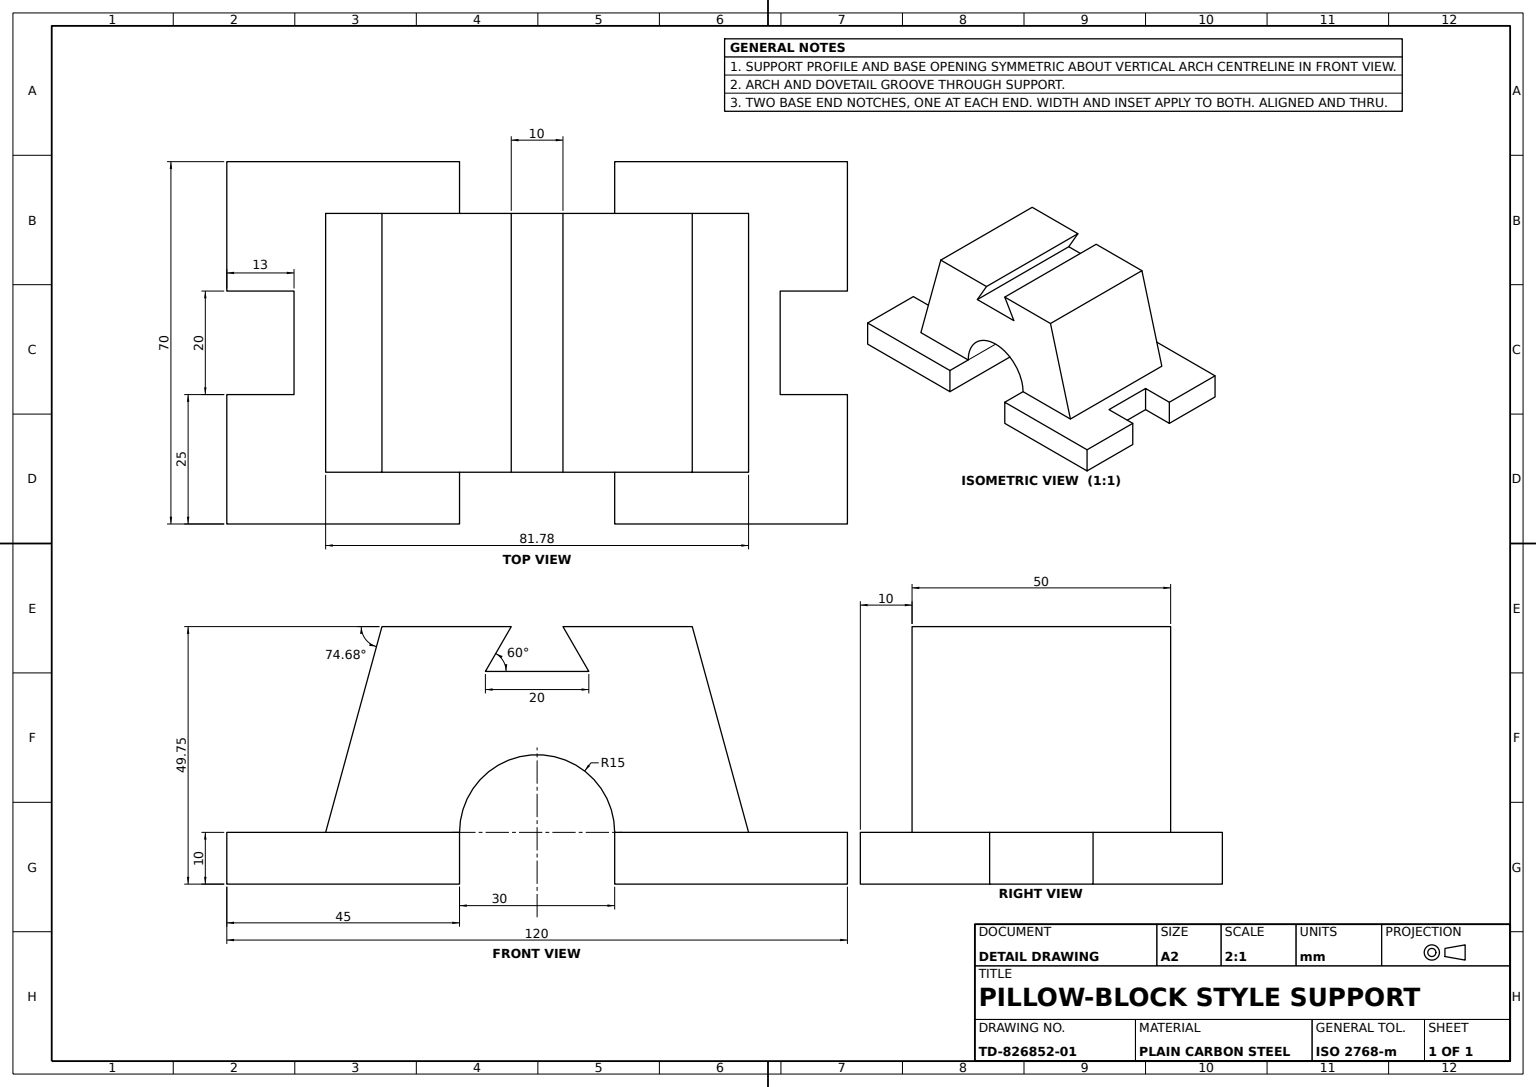
from build123d import *

# Parameters (mm, degrees)
BASE_PLATE_10MM_DEPTH         = 10
SUPPORT_BLOCK_50MM_DEPTH      = 25
SUPPORT_BLOCK_50MM_DEPTH_BACK = 25
ARCH_THROUGH_CUT_DEPTH        = 35
ARCH_THROUGH_CUT_DEPTH_BACK   = 35
UPPER_BOSS_SKETCH_W           = 20
UPPER_BOSS_SKETCH_H           = 10
UPPER_BOSS_3MM_DEPTH          = 3
BASE_PAD_SKETCH_W             = 20
BASE_PAD_SKETCH_H             = 10
BASE_PAD_4_19MM_DEPTH         = 4.19


with BuildPart() as part:
    # Base Plate Sketch → Base Plate 10mm (new body)
    with BuildSketch(Plane(origin=(0, 0, 0), x_dir=(1, 0, 0), z_dir=(0, 1, 0))):
        Polygon((60, 10), (42.8083356, 10), (42.8083356, -10), (60, -10), (60, -35), (-60, -35), (-60, -10), (-44.9850804, -10), (-44.9850804, 10), (-60, 10), (-60, 35), (60, 35), align=None)
    extrude(amount=BASE_PLATE_10MM_DEPTH)

    # Support Block Profile → Support Block 50mm (add, two sides: drawn at the far end of the back side and taken through both)
    with BuildSketch(Plane.XY.offset(-SUPPORT_BLOCK_50MM_DEPTH_BACK)):
        with BuildLine():
            Line((-40.889682702, 10), (-15, 10))
            ThreePointArc((-15, 10), (0, 25), (15, 10))
            Line((15, 10), (40.889682702, 10))
            Line((40.889682702, 10), (30, 49.749371855))
            Line((30, 49.749371855), (5, 49.749371855))
            Line((5, 49.749371855), (10, 41.089117817))
            Line((10, 41.089117817), (-10, 41.089117817))
            Line((-10, 41.089117817), (-5, 49.749371855))
            Line((-5, 49.749371855), (-30, 49.749371855))
            Line((-30, 49.749371855), (-40.889682702, 10))
        make_face()
        with BuildLine():
            ThreePointArc((15, 10), (0, 25), (-15, 10))
            Line((-15, 10), (0, 10))
            Line((0, 10), (15, 10))
        make_face()
    extrude(amount=SUPPORT_BLOCK_50MM_DEPTH + SUPPORT_BLOCK_50MM_DEPTH_BACK)

    # Arch Cut Sketch → Arch Through Cut (cut, two sides: drawn at the far end of the back side and taken through both)
    with BuildSketch(Plane.XY.offset(-ARCH_THROUGH_CUT_DEPTH_BACK)):
        with BuildLine():
            Line((-15, 10), (-15, 0))
            Line((-15, 0), (15, 0))
            Line((15, 0), (15, 10))
            ThreePointArc((15, 10), (0, 25), (-15, 10))
        make_face()
    extrude(amount=ARCH_THROUGH_CUT_DEPTH + ARCH_THROUGH_CUT_DEPTH_BACK, mode=Mode.SUBTRACT)

    # Upper Boss Sketch → Upper Boss 3mm (add)
    with BuildSketch(Plane(origin=(-44, 0, 0), x_dir=(0, 0, -1), z_dir=(1, 0, 0))):
        with Locations((0, 5)):
            Rectangle(UPPER_BOSS_SKETCH_W, UPPER_BOSS_SKETCH_H)
    extrude(amount=-UPPER_BOSS_3MM_DEPTH)

    # Base Pad Sketch → Base Pad 4.19mm (add)
    with BuildSketch(Plane(origin=(42.8083356, 0, 0), x_dir=(0, 0, -1), z_dir=(1, 0, 0))):
        with Locations((0, 5)):
            Rectangle(BASE_PAD_SKETCH_W, BASE_PAD_SKETCH_H)
    extrude(amount=BASE_PAD_4_19MM_DEPTH)


solid = part.part
